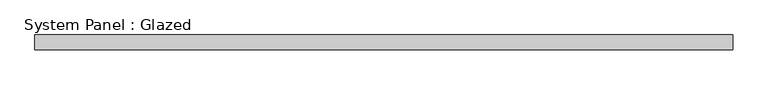
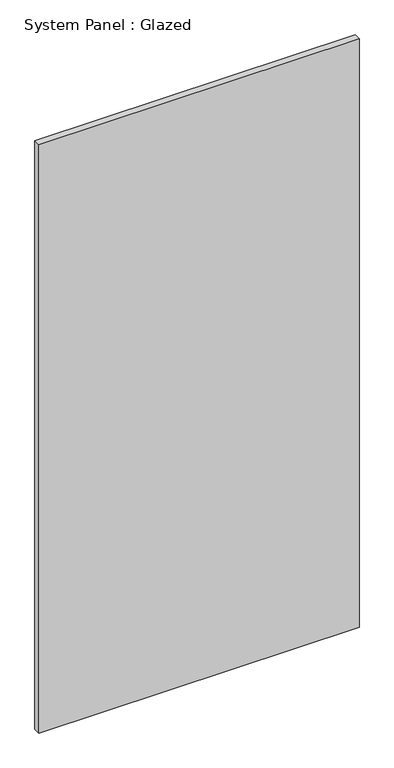
"""IFC4 building model written with IfcOpenShell, lengths in millimetres: plate geometry, System Panel : Glazed."""

from ifc_helpers import new_model, si_unit, origin, origin_with_axes, place, context, project, spatial, polyline, outline, extrude, source, transform, mapped, element, save


def system_panel_glazed_153d3200(model_context):
    return source(origin(), model_context, "Body", "SweptSolid", [
        extrude(outline(polyline([(603.2499999, 19.05), (-603.2499999, 19.05), (-603.2499999, 44.45), (603.2499999, 44.45), (603.2499999, 19.05)])), origin_with_axes(), (0.0, 0.0, 1.0), 2343.15),
    ])


if __name__ == "__main__":
    model = new_model("IFC4")
    model_context = context("Model", 3, world=origin())
    ifc_project = project(units=[si_unit("LENGTHUNIT", "METRE", prefix="MILLI")], contexts=[model_context])
    site = spatial("IfcSite", under=ifc_project)
    building = spatial("IfcBuilding", under=site)
    placement = place(None, origin())
    system_panel_glazed_shape = system_panel_glazed_153d3200(model_context)
    element("IfcPlate", 1, ObjectType="System Panel : Glazed", at=placement, inside=building, context=model_context, shape_type="MappedRepresentation", body=[
        mapped(system_panel_glazed_shape, transform((0.0, 0.0, 0.0), x_axis=(1.0, 0.0, 0.0), y_axis=(0.0, 1.0, 0.0), z_axis=(0.0, 0.0, 1.0))),
    ])
    save(model, "model.ifc")

# Revit data of these elements
# Type "System Panel : Glazed"
#   Construction Type Id = "GSP4R"
#   Analytic Construction = "1/8 in Pilkington single glazing"
#   Visual Light Transmittance = 0.9
#   Solar Heat Gain Coefficient = 0.86
#   Heat Transfer Coefficient (U) = 1.18115 BTU/(h·ft²·°F)
#   Define Thermal Properties by = 1
# Element 1 (IfcPlate, "System Panel : Glazed")
#   Materials on its faces: "Glass"
# Materials
#   "Glass": class "Glass", colour RGB 0 128 192, transparency 0.75, Description = "Soda Lime Glass", Cost = 0
